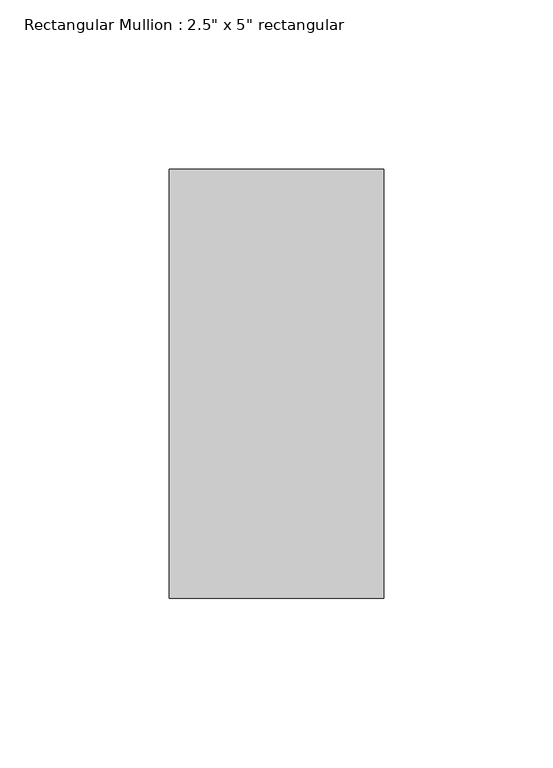
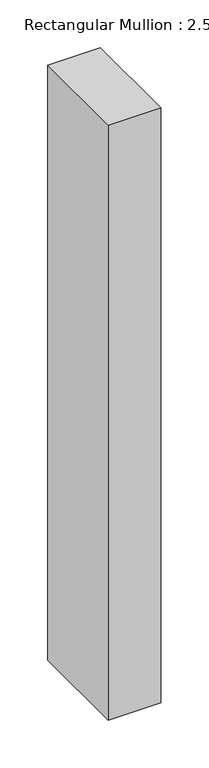
"""IFC4 building model written with IfcOpenShell, lengths in millimetres: member geometry."""

from ifc_helpers import new_model, si_unit, frame, origin, place, context, project, spatial, polyline, outline, extrude, source, transform, mapped, element, save


def member_ee585a1e(model_context):
    return source(origin(), model_context, "Body", "SweptSolid", [
        extrude(outline(polyline([(0.0, 63.5), (0.0, -63.5), (-63.5, -63.5), (-63.5, 63.5), (0.0, 63.5)])), frame((0.0, 0.0, -760.850254), z_axis=(0.0, 0.0, 1.0), x_axis=(1.0, 0.0, 0.0)), (0.0, 0.0, 1.0), 760.850254),
    ])


if __name__ == "__main__":
    model = new_model("IFC4")
    model_context = context("Model", 3, world=origin())
    ifc_project = project(units=[si_unit("LENGTHUNIT", "METRE", prefix="MILLI")], contexts=[model_context])
    site = spatial("IfcSite", under=ifc_project)
    building = spatial("IfcBuilding", under=site)
    placement = place(None, origin())
    member_shape = member_ee585a1e(model_context)
    element("IfcMember", 1, ObjectType="Rectangular Mullion : 2.5\" x 5\" rectangular", at=placement, inside=building, context=model_context, shape_type="MappedRepresentation", body=[
        mapped(member_shape, transform((0.0, 0.0, 0.0), x_axis=(1.0, 0.0, 0.0), y_axis=(0.0, 1.0, 0.0), z_axis=(0.0, 0.0, 1.0))),
    ])
    save(model, "model.ifc")

# Revit data of these elements
# Type "Rectangular Mullion : 2.5\" x 5\" rectangular"
#   built-in parameter 1007304 = 0.416667 (stored number, unit not read)
#   built-in parameter 1007301 = 0.104167 (stored number, unit not read)
#   built-in parameter 1007300 = 0.104167 (stored number, unit not read)
# Element 1 (IfcMember, "Rectangular Mullion : 2.5\" x 5\" rectangular")
#   Materials on its faces: "Aluminum"
# Materials
#   "Aluminum": class "Metal", colour RGB 247 247 247, transparency 0, Description = "Aluminum 6061", Cost = 0
